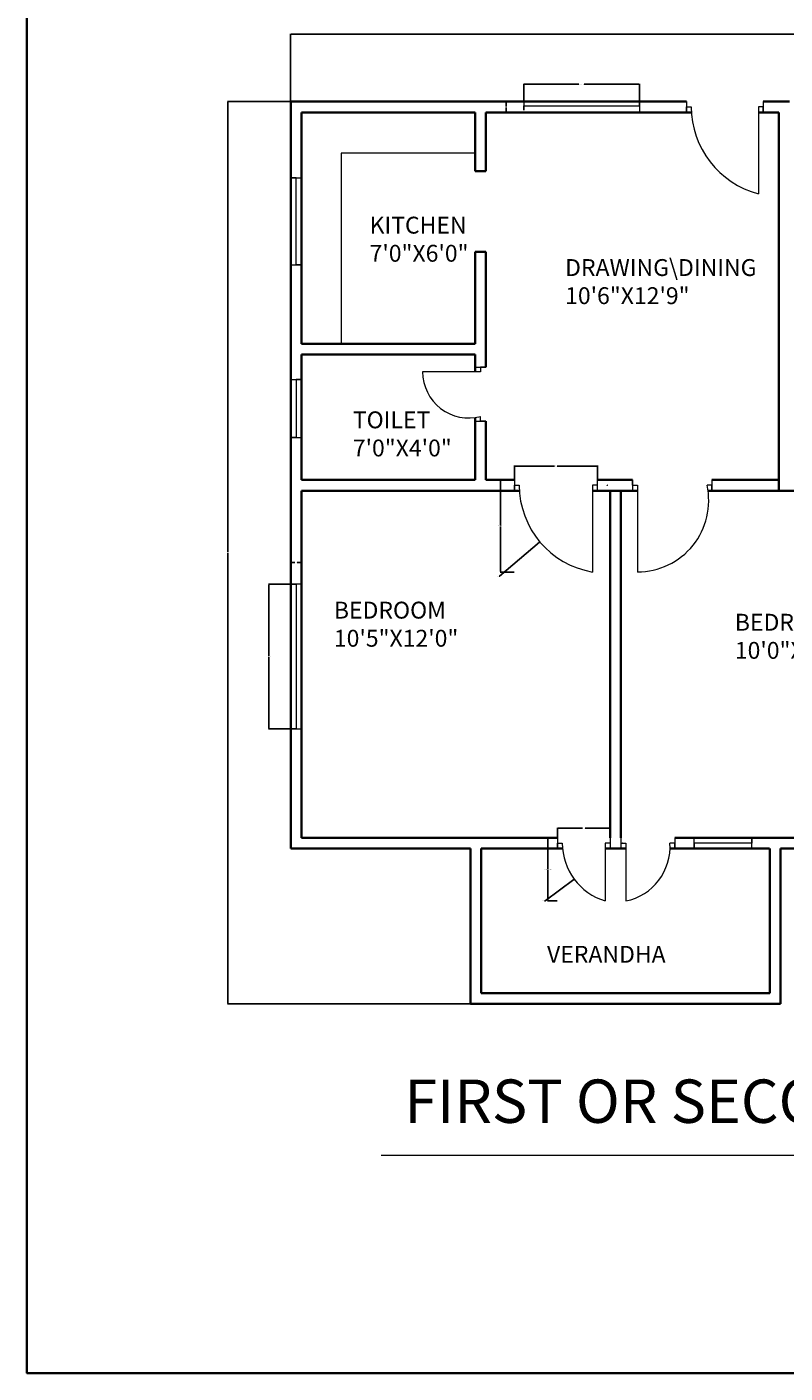
# Model space of a CAD drawing. Units: inches. Extents: x 2055 to 3558, y 1520 to 2888.
# Tile 1 of 8: x 2055 to 2369, y 1520 to 2079. Entities that reach past the tile are written whole.
import ezdxf

# ---------------------------------------------------------------- set-up
doc = ezdxf.new("R2010")
doc.units = ezdxf.units.IN
for name, color, linetype, lineweight in [('A-ANNO-DIMS', 2, 'Continuous', 18), ('A-ANNO-TEXT', 7, 'Continuous', 18), ('A-ANNO-TTLB', 7, 'Continuous', 35), ('A-AREA-IDEN', 7, 'Continuous', 18), ('A-DOOR', 3, 'Continuous', 18), ('A-FLOR-FIXT', 8, 'Continuous', 18), ('A-GLAZ', 4, 'Continuous', 18), ('A-WALL', 7, 'Continuous', 35)]:
    doc.layers.add(name, color=color, linetype=linetype, lineweight=lineweight)
doc.styles.get("Standard").update_dxf_attribs({"font": 'arial.ttf'})
doc.dimstyles.get("Standard").update_dxf_attribs({"dimtxt": 0.18, "dimasz": 0.18, "dimexe": 0.18, "dimexo": 0.0625, "dimgap": 0.09, "dimtad": 0, "dimtih": 1, "dimtoh": 1, "dimdec": 4, "dimzin": 0, "dimdsep": 46, "dimtxsty": 'Standard', "dimcen": 0.09, "dimadec": 0, "dimazin": 0, "dimtfac": 1, "dimtdec": 4, "dimtofl": 0, "dimtmove": 0, "dimatfit": 3, "dimfxl": 1, "dimtolj": 1, "dimtzin": 0, "dimarcsym": 0})

# ---------------------------------------------------------------- blocks, each defined once
blk = doc.blocks.new('DOOR-ENTRY-36-C')
for p, q in [((0, 38.25), (0, 33.75)), ((0, 33.75), (0, 36)), ((0, 36), (2, 36)), ((31.88, 36), (29.88, 36)), ((29.88, 36), (29.88, 0)), ((31.88, 38.25), (31.88, 33.75)), ((31.88, 33.75), (31.88, 36))]:
    blk.add_line(p, q)
blk.add_arc((39.18, 36), 37.18, 180, 255.5126)
blk = doc.blocks.new('DOOR-BATH-24-C')
for p, q in [((21.75, 22.46), (26.25, 22.46)), ((26.25, 22.46), (24, 22.46)), ((24, 22.46), (24, 20.46)), ((24, 20.46), (0, 20.46)), ((24, 0), (24, 2)), ((21.75, 0), (26.25, 0)), ((26.25, 0), (24, 0))]:
    blk.add_line(p, q)
blk.add_arc((19.1, 20.46), 19.1, 180, 284.8648)
blk = doc.blocks.new('DOOR-BED-36-D')
for p, q in [((0.16, 33.75), (0, 38.25)), ((0, 38.25), (0.08, 36)), ((0.08, 36), (2.08, 36)), ((2.08, 36), (2.08, 0)), ((33, 36), (31, 36)), ((33, 38.25), (33, 33.75)), ((33, 33.75), (33, 36))]:
    blk.add_line(p, q)
blk.add_arc((2.08, 29.62), 29.61, 270, 12.4519)
blk = doc.blocks.new('DOOR-BED-36-E')
for p, q in [((0, 38.25), (0, 33.75)), ((0, 33.75), (0, 36)), ((0, 36), (2, 36)), ((34.42, 36), (32.42, 36)), ((32.42, 36), (32.42, 0)), ((34.42, 33.75), (34.42, 38.25))]:
    blk.add_line(p, q)
blk.add_arc((38.51, 36), 36.51, 180, 260.3872)
blk = doc.blocks.new('DOOR-VERANDA-24-C')
for p, q in [((0, 26.25), (0, 21.75)), ((0, 21.75), (0, 24)), ((0, 24), (2, 24)), ((21.82, 24), (19.82, 24)), ((19.82, 24), (19.82, 0)), ((21.82, 26.25), (21.82, 21.75))]:
    blk.add_line(p, q)
blk.add_arc((27.07, 24), 25.07, 180, 253.1988)
blk = doc.blocks.new('DOOR-VERANDA-24-D')
for p, q in [((0, 26.25), (0, 21.75)), ((0, 24), (2, 24)), ((2, 24), (2, 0)), ((22.33, 24), (20.33, 24)), ((22.33, 26.25), (22.33, 21.75)), ((22.33, 21.75), (22.33, 24))]:
    blk.add_line(p, q)
blk.add_arc((-2.55, 22.48), 22.94, 281.4505, 3.8037)
blk = doc.blocks.new('WIN-36')
for p, q in [((2.25, 36), (0, 36)), ((0, 36), (4.5, 36)), ((2.25, 0), (2.25, 36)), ((0, 0), (4.5, 0)), ((4.5, 0), (2.25, 0))]:
    blk.add_line(p, q)
blk = doc.blocks.new('WIN-24')
for p, q in [((0, 24), (4.5, 24)), ((4.5, 24), (2.25, 24)), ((2.25, 24), (2.25, 0)), ((2.25, 0), (0, 0)), ((0, 0), (4.5, 0))]:
    blk.add_line(p, q)
blk = doc.blocks.new('WIN-60-2')
for p, q in [((4.5, 60), (0, 60)), ((0, 60), (2.25, 60)), ((2.25, 60), (2.25, 0)), ((2.25, 0), (0, 0)), ((0, 0), (4.5, 0))]:
    blk.add_line(p, q)
blk = doc.blocks.new('WIN-48-2')
for p, q in [((0, 4.5), (0, 0.97)), ((0, 0.97), (0, 2.74)), ((0, 2.74), (48, 2.74)), ((48, 2.74), (48, 4.5)), ((48, 4.5), (48, 0))]:
    blk.add_line(p, q)
blk = doc.blocks.new('COUNTER-3')
for p, q in [((55.49, 79.01), (0, 79.01)), ((0, 79.01), (0, 0))]:
    blk.add_line(p, q)
blk = doc.blocks.new('VERANDA-PERIMETER')
for p, q in [((0, 0), (0, 64.5)), ((4.5, 64.5), (4.5, 4.5)), ((124.15, 4.5), (124.15, 64.5)), ((128.65, 64.5), (128.65, 4.5)), ((4.5, 0), (0, 0)), ((4.5, 4.5), (124.15, 4.5)), ((128.65, 0), (4.5, 0)), ((128.65, 4.5), (128.65, 0))]:
    blk.add_line(p, q)
blk = doc.blocks.new('*D48')
at = {"layer": 'A-ANNO-DIMS', "color": 0, "lineweight": -2, "transparency": 16777216}
for p, q in [((2164.11, 1847.67), (2154.99, 1847.67)), ((2155.17, 1847.49), (2155.17, 1817.85)), ((2155.17, 1787.85), (2155.17, 1817.48)), ((2164.11, 1787.67), (2154.99, 1787.67))]:
    blk.add_line(p, q, dxfattribs=at)
at = {"layer": 'A-ANNO-DIMS', "color": 0, "transparency": 16777216}
for points in [[(2155.14, 1847.49), (2155.2, 1847.49), (2155.17, 1847.67)], [(2155.14, 1787.85), (2155.2, 1787.85), (2155.17, 1787.67)]]:
    blk.add_solid(points, dxfattribs=at)
at = {"layer": 'Defpoints', "color": 0, "transparency": 16777216}
for p in [(2155.17, 1847.67), (2164.17, 1847.67), (2164.17, 1787.67)]:
    blk.add_point(p, dxfattribs=at)
at = {"layer": 'A-ANNO-DIMS', "color": 0, "transparency": 16777216, "insert": (2155.17, 1817.67), "char_height": 0.18, "attachment_point": 5}
blk.add_mtext('\\A1;WINDOW 60 TYP.', dxfattribs=at)
blk = doc.blocks.new('*D49')
at = {"layer": 'A-ANNO-DIMS', "color": 0, "lineweight": -2, "transparency": 16777216}
for p, q in [((2164.17, 1847.73), (2164.17, 1856.85)), ((2164.35, 1856.67), (2165.97, 1856.67)), ((2168.49, 1856.67), (2166.88, 1856.67)), ((2168.67, 1847.73), (2168.67, 1856.85))]:
    blk.add_line(p, q, dxfattribs=at)
at = {"layer": 'A-ANNO-DIMS', "color": 0, "transparency": 16777216}
for points in [[(2164.35, 1856.7), (2164.35, 1856.64), (2164.17, 1856.67)], [(2168.49, 1856.7), (2168.49, 1856.64), (2168.67, 1856.67)]]:
    blk.add_solid(points, dxfattribs=at)
at = {"layer": 'Defpoints', "color": 0, "transparency": 16777216}
for p in [(2168.67, 1856.67), (2164.17, 1847.67), (2168.67, 1847.67)]:
    blk.add_point(p, dxfattribs=at)
at = {"layer": 'A-ANNO-DIMS', "color": 0, "transparency": 16777216, "insert": (2166.42, 1856.67), "char_height": 0.18, "attachment_point": 5}
blk.add_mtext('\\A1;5 TYP.', dxfattribs=at)
blk = doc.blocks.new('*D76')
at = {"layer": 'A-ANNO-DIMS', "color": 0, "lineweight": -2, "transparency": 16777216}
for p, q in [((2256.93, 1891), (2251.07, 1891)), ((2251.25, 1890.82), (2251.25, 1872.06)), ((2251.25, 1852.93), (2251.25, 1871.69)), ((2256.93, 1852.75), (2251.07, 1852.75))]:
    blk.add_line(p, q, dxfattribs=at)
at = {"layer": 'A-ANNO-DIMS', "color": 0, "transparency": 16777216}
for points in [[(2251.22, 1890.82), (2251.28, 1890.82), (2251.25, 1891)], [(2251.22, 1852.93), (2251.28, 1852.93), (2251.25, 1852.75)]]:
    blk.add_solid(points, dxfattribs=at)
at = {"layer": 'Defpoints', "color": 0, "transparency": 16777216}
for p in [(2251.25, 1891), (2256.99, 1891), (2256.99, 1852.75)]:
    blk.add_point(p, dxfattribs=at)
at = {"layer": 'A-ANNO-DIMS', "color": 0, "transparency": 16777216, "insert": (2251.25, 1871.87), "char_height": 0.18, "attachment_point": 5}
blk.add_mtext('\\A1;BED DOOR 38 TYP.', dxfattribs=at)
blk = doc.blocks.new('*D77')
at = {"layer": 'A-ANNO-DIMS', "color": 0, "lineweight": -2, "transparency": 16777216}
for p, q in [((2256.99, 1891.06), (2256.99, 1896.92)), ((2257.17, 1896.74), (2273.67, 1896.74)), ((2291.23, 1896.74), (2274.73, 1896.74)), ((2291.41, 1891.06), (2291.41, 1896.92))]:
    blk.add_line(p, q, dxfattribs=at)
at = {"layer": 'A-ANNO-DIMS', "color": 0, "transparency": 16777216}
for points in [[(2257.17, 1896.77), (2257.17, 1896.71), (2256.99, 1896.74)], [(2291.23, 1896.77), (2291.23, 1896.71), (2291.41, 1896.74)]]:
    blk.add_solid(points, dxfattribs=at)
at = {"layer": 'Defpoints', "color": 0, "transparency": 16777216}
for p in [(2291.41, 1896.74), (2256.99, 1891), (2291.41, 1891)]:
    blk.add_point(p, dxfattribs=at)
at = {"layer": 'A-ANNO-DIMS', "color": 0, "transparency": 16777216, "insert": (2274.2, 1896.74), "char_height": 0.18, "attachment_point": 5}
blk.add_mtext('\\A1;34 TYP.', dxfattribs=at)
blk = doc.blocks.new('*D86')
at = {"layer": 'A-ANNO-DIMS', "color": 0, "lineweight": -2, "transparency": 16777216}
for p, q in [((2274.79, 1742.5), (2270.73, 1742.5)), ((2270.91, 1742.32), (2270.91, 1729.56)), ((2270.91, 1716.43), (2270.91, 1729.19)), ((2274.79, 1716.25), (2270.73, 1716.25))]:
    blk.add_line(p, q, dxfattribs=at)
at = {"layer": 'A-ANNO-DIMS', "color": 0, "transparency": 16777216}
for points in [[(2270.88, 1742.32), (2270.94, 1742.32), (2270.91, 1742.5)], [(2270.88, 1716.43), (2270.94, 1716.43), (2270.91, 1716.25)]]:
    blk.add_solid(points, dxfattribs=at)
at = {"layer": 'Defpoints', "color": 0, "transparency": 16777216}
for p in [(2270.91, 1742.5), (2274.85, 1742.5), (2274.85, 1716.25)]:
    blk.add_point(p, dxfattribs=at)
at = {"layer": 'A-ANNO-DIMS', "color": 0, "transparency": 16777216, "insert": (2270.91, 1729.37), "char_height": 0.18, "attachment_point": 5}
blk.add_mtext('\\A1;VERANDA DOOR 26 TYP.', dxfattribs=at)
blk = doc.blocks.new('*D87')
at = {"layer": 'A-ANNO-DIMS', "color": 0, "lineweight": -2, "transparency": 16777216}
for p, q in [((2274.85, 1742.56), (2274.85, 1746.62)), ((2275.03, 1746.44), (2285.23, 1746.44)), ((2296.49, 1746.44), (2286.29, 1746.44)), ((2296.67, 1742.56), (2296.67, 1746.62))]:
    blk.add_line(p, q, dxfattribs=at)
at = {"layer": 'A-ANNO-DIMS', "color": 0, "transparency": 16777216}
for points in [[(2275.03, 1746.47), (2275.03, 1746.41), (2274.85, 1746.44)], [(2296.49, 1746.47), (2296.49, 1746.41), (2296.67, 1746.44)]]:
    blk.add_solid(points, dxfattribs=at)
at = {"layer": 'Defpoints', "color": 0, "transparency": 16777216}
for p in [(2296.67, 1746.44), (2274.85, 1742.5), (2296.67, 1742.5)]:
    blk.add_point(p, dxfattribs=at)
at = {"layer": 'A-ANNO-DIMS', "color": 0, "transparency": 16777216, "insert": (2285.76, 1746.44), "char_height": 0.18, "attachment_point": 5}
blk.add_mtext('\\A1;22 TYP.', dxfattribs=at)
blk = doc.blocks.new('*D104')
at = {"layer": 'A-ANNO-DIMS', "color": 0, "lineweight": -2, "transparency": 16777216}
for p, q in [((2260.84, 2048.06), (2260.84, 2055.38)), ((2261.02, 2055.2), (2283.72, 2055.2)), ((2308.66, 2055.2), (2285.96, 2055.2)), ((2308.84, 2048.06), (2308.84, 2055.38))]:
    blk.add_line(p, q, dxfattribs=at)
at = {"layer": 'A-ANNO-DIMS', "color": 0, "transparency": 16777216}
for points in [[(2261.02, 2055.23), (2261.02, 2055.17), (2260.84, 2055.2)], [(2308.66, 2055.23), (2308.66, 2055.17), (2308.84, 2055.2)]]:
    blk.add_solid(points, dxfattribs=at)
at = {"layer": 'Defpoints', "color": 0, "transparency": 16777216}
for p in [(2308.84, 2055.2), (2260.84, 2048), (2308.84, 2048)]:
    blk.add_point(p, dxfattribs=at)
at = {"layer": 'A-ANNO-DIMS', "color": 0, "transparency": 16777216, "insert": (2284.84, 2055.2), "char_height": 0.18, "attachment_point": 5}
blk.add_mtext('\\A1;WINDOW 48 TYP.', dxfattribs=at)
blk = doc.blocks.new('*D105')
at = {"layer": 'A-ANNO-DIMS', "color": 0, "lineweight": -2, "transparency": 16777216}
for p, q in [((2260.77, 2048), (2253.46, 2048)), ((2253.64, 2047.82), (2253.64, 2045.93)), ((2253.64, 2043.68), (2253.64, 2045.57)), ((2260.77, 2043.5), (2253.46, 2043.5))]:
    blk.add_line(p, q, dxfattribs=at)
at = {"layer": 'A-ANNO-DIMS', "color": 0, "transparency": 16777216}
for points in [[(2253.61, 2047.82), (2253.67, 2047.82), (2253.64, 2048)], [(2253.61, 2043.68), (2253.67, 2043.68), (2253.64, 2043.5)]]:
    blk.add_solid(points, dxfattribs=at)
at = {"layer": 'Defpoints', "color": 0, "transparency": 16777216}
for p in [(2253.64, 2048), (2260.84, 2048), (2260.84, 2043.5)]:
    blk.add_point(p, dxfattribs=at)
at = {"layer": 'A-ANNO-DIMS', "color": 0, "transparency": 16777216, "insert": (2253.64, 2045.75), "char_height": 0.18, "attachment_point": 5}
blk.add_mtext('\\A1;5 TYP.', dxfattribs=at)
blk = doc.blocks.new('*D121')
at = {"layer": 'A-ANNO-DIMS', "color": 0, "lineweight": -2, "transparency": 16777216}
for p, q in [((2164.17, 2048.06), (2164.17, 2076.13)), ((2164.35, 2075.95), (2420.03, 2075.95)), ((2676.49, 2075.95), (2420.82, 2075.95)), ((2676.67, 2048.06), (2676.67, 2076.13))]:
    blk.add_line(p, q, dxfattribs=at)
at = {"layer": 'A-ANNO-DIMS', "color": 0, "transparency": 16777216}
for points in [[(2164.35, 2075.98), (2164.35, 2075.92), (2164.17, 2075.95)], [(2676.49, 2075.98), (2676.49, 2075.92), (2676.67, 2075.95)]]:
    blk.add_solid(points, dxfattribs=at)
at = {"layer": 'Defpoints', "color": 0, "transparency": 16777216}
for p in [(2676.67, 2075.95), (2164.17, 2048), (2676.67, 2048)]:
    blk.add_point(p, dxfattribs=at)
at = {"layer": 'A-ANNO-DIMS', "color": 0, "transparency": 16777216, "insert": (2420.42, 2075.95), "char_height": 0.18, "attachment_point": 5}
blk.add_mtext('\\A1;512.5', dxfattribs=at)
blk = doc.blocks.new('*D122')
at = {"layer": 'A-ANNO-DIMS', "color": 0, "lineweight": -2, "transparency": 16777216}
for p, q in [((2164.11, 2048), (2137.94, 2048)), ((2138.12, 2047.82), (2138.12, 1860.93)), ((2138.12, 1673.68), (2138.12, 1860.57)), ((2238.68, 1673.5), (2137.94, 1673.5))]:
    blk.add_line(p, q, dxfattribs=at)
at = {"layer": 'A-ANNO-DIMS', "color": 0, "transparency": 16777216}
for points in [[(2138.09, 2047.82), (2138.15, 2047.82), (2138.12, 2048)], [(2138.09, 1673.68), (2138.15, 1673.68), (2138.12, 1673.5)]]:
    blk.add_solid(points, dxfattribs=at)
at = {"layer": 'Defpoints', "color": 0, "transparency": 16777216}
for p in [(2164.17, 2048), (2138.12, 1673.5), (2238.74, 1673.5)]:
    blk.add_point(p, dxfattribs=at)
at = {"layer": 'A-ANNO-DIMS', "color": 0, "transparency": 16777216, "insert": (2138.12, 1860.75), "char_height": 0.18, "attachment_point": 5}
blk.add_mtext('\\A1;374.5', dxfattribs=at)
blk = doc.blocks.new('*D174')
at = {"layer": 'A-ANNO-DIMS', "color": 0, "lineweight": -2, "transparency": 16777216}
for p, q in [((2295.41, 1888.75), (2295.59, 1888.75)), ((2295.5, 1888.66), (2295.5, 1888.84)), ((2250.88, 1851.05), (2267.47, 1865.07)), ((2250.7, 1851.05), (2250.88, 1851.05))]:
    blk.add_line(p, q, dxfattribs=at)
at = {"layer": 'A-ANNO-DIMS', "color": 0, "transparency": 16777216}
blk.add_solid([(2267.46, 1865.09), (2267.49, 1865.05), (2267.61, 1865.18)], dxfattribs=at)
at = {"layer": 'Defpoints', "color": 0, "transparency": 16777216}
for p in [(2295.5, 1888.75), (2267.61, 1865.18)]:
    blk.add_point(p, dxfattribs=at)
at = {"layer": 'A-ANNO-DIMS', "color": 0, "transparency": 16777216, "insert": (2250.24, 1851.05), "char_height": 0.18, "attachment_point": 5}
blk.add_mtext('\\A1;R36.51', dxfattribs=at)
blk = doc.blocks.new('*D180')
at = {"layer": 'A-ANNO-DIMS', "color": 0, "lineweight": -2, "transparency": 16777216}
for p, q in [((2301.83, 1740.25), (2302.01, 1740.25)), ((2301.92, 1740.16), (2301.92, 1740.34)), ((2269.72, 1716.33), (2281.65, 1725.19)), ((2269.54, 1716.33), (2269.72, 1716.33))]:
    blk.add_line(p, q, dxfattribs=at)
at = {"layer": 'A-ANNO-DIMS', "color": 0, "transparency": 16777216}
blk.add_solid([(2281.63, 1725.22), (2281.67, 1725.17), (2281.79, 1725.3)], dxfattribs=at)
at = {"layer": 'Defpoints', "color": 0, "transparency": 16777216}
for p in [(2301.92, 1740.25), (2281.79, 1725.3)]:
    blk.add_point(p, dxfattribs=at)
at = {"layer": 'A-ANNO-DIMS', "color": 0, "transparency": 16777216, "insert": (2269.06, 1716.33), "char_height": 0.18, "attachment_point": 5}
blk.add_mtext('\\A1;R25.07', dxfattribs=at)

msp = doc.modelspace()

# ---------------------------------------------------------------- linework, layer by layer
at = {"layer": 'A-ANNO-TEXT'}
msp.add_line((2201.7713, 1610.7234), (2548.8845, 1610.7234), dxfattribs=at)
at = {"layer": 'A-ANNO-TTLB'}
msp.add_lwpolyline([(2054.7598, 2888.2545), (3557.8479, 2888.2545), (3557.8479, 1520.3256), (2054.7598, 1520.3256)], close=True, dxfattribs=at)
at = {"layer": 'A-WALL'}
for p, q in [((2164.1747, 2047.9995), (2328.3753, 2047.9995)), ((2164.1747, 2047.9995), (2164.1747, 1737.9995)), ((2360.2558, 2047.9995), (2371.1747, 2047.9995)), ((2168.6747, 2043.4995), (2168.6747, 1947.4995)), ((2168.6747, 2043.4995), (2240.6747, 2043.4995)), ((2240.6747, 2043.4995), (2240.6747, 2019.1081)), ((2245.1747, 2043.4995), (2245.1747, 2019.1081)), ((2245.1747, 2043.4995), (2330.4434, 2043.4995)), ((2358.2558, 2043.4995), (2366.6747, 2043.4995)), ((2366.6747, 2043.4995), (2366.6747, 1947.4995)), ((2366.6747, 2043.4995), (2366.6747, 1886.4995)), ((2240.6747, 2019.1081), (2245.1747, 2019.1081)), ((2245.1747, 1985.6374), (2240.6747, 1985.6374)), ((2240.6747, 1985.6374), (2240.6747, 1947.4995)), ((2245.1747, 1985.6374), (2245.1747, 1937.7895)), ((2168.6747, 1947.4995), (2240.6747, 1947.4995)), ((2168.6747, 1942.9995), (2240.6747, 1942.9995)), ((2168.6747, 1942.9995), (2168.6747, 1890.9995)), ((2240.6747, 1942.9995), (2240.6747, 1935.7895)), ((2240.6747, 1916.8741), (2240.6747, 1890.9995)), ((2245.1747, 1915.3286), (2245.1747, 1890.9995)), ((2168.6747, 1890.9995), (2240.6747, 1890.9995)), ((2245.1747, 1890.9995), (2256.9898, 1890.9995)), ((2291.4053, 1890.9995), (2305.9247, 1890.9995)), ((2338.9237, 1890.9995), (2366.6747, 1890.9995)), ((2168.6747, 1886.4995), (2259.0592, 1886.4995)), ((2168.6747, 1886.4995), (2168.6747, 1742.4995)), ((2245.1747, 1886.4995), (2259.0592, 1886.4995)), ((2289.4053, 1886.4995), (2308.0058, 1886.4995)), ((2289.4053, 1886.4995), (2308.0058, 1886.4995)), ((2296.6747, 1886.4995), (2296.6747, 1742.4995)), ((2301.1747, 1886.4995), (2301.1747, 1742.4995)), ((2337.3301, 1886.4995), (2366.6747, 1886.4995)), ((2337.3301, 1886.4995), (2422.6747, 1886.4995)), ((2164.1747, 1737.9995), (2238.745, 1737.9995)), ((2168.6747, 1742.4995), (2274.8511, 1742.4995)), ((2243.245, 1737.9995), (2276.9523, 1737.9995)), ((2245.1747, 1742.4995), (2274.8511, 1742.4995)), ((2294.6747, 1737.9995), (2303.1747, 1737.9995)), ((2321.545, 1737.9995), (2362.8911, 1737.9995)), ((2323.5061, 1742.4995), (2508.8547, 1742.4995)), ((2323.5061, 1742.4995), (2366.6747, 1742.4995)), ((2367.3911, 1737.9995), (2422.6747, 1737.9995))]:
    msp.add_line(p, q, dxfattribs=at)

# ---------------------------------------------------------------- block references
at = {"layer": 'A-DOOR'}
for name, p in [('DOOR-ENTRY-36-C', (2328.375, 2009.749)), ('DOOR-BATH-24-C', (2218.925, 1915.329)), ('DOOR-BED-36-E', (2256.99, 1852.749)), ('DOOR-BED-36-D', (2305.925, 1852.749)), ('DOOR-VERANDA-24-C', (2274.851, 1716.249)), ('DOOR-VERANDA-24-D', (2301.175, 1716.249))]:
    msp.add_blockref(name, p, dxfattribs=at)
at = {"layer": 'A-FLOR-FIXT'}
msp.add_blockref('COUNTER-3', (2185.186, 1947.499), dxfattribs=at)
at = {"layer": 'A-GLAZ'}
for name, p in [('WIN-48-2', (2260.837, 2043.499)), ('WIN-36', (2164.175, 1980.291)), ('WIN-24', (2164.175, 1908.63)), ('WIN-60-2', (2164.175, 1787.665))]:
    msp.add_blockref(name, p, dxfattribs=at)
at = {"layer": 'A-GLAZ', "extrusion": (0, 0, -1), "zscale": -1, "rotation": 90}
msp.add_blockref('WIN-24', (-2331.5394, 1737.9998), dxfattribs=at)
at = {"layer": 'A-WALL'}
msp.add_blockref('VERANDA-PERIMETER', (2238.745, 1673.499), dxfattribs=at)

# ---------------------------------------------------------------- texts
at = {"layer": 'A-ANNO-TEXT', "insert": (2211.3331, 1642.1482), "char_height": 18, "attachment_point": 1}
msp.add_mtext_dynamic_manual_height_columns('FIRST OR SECOND FLOOR ', width=532.043788, gutter_width=12.5, heights=[0], dxfattribs=at)
at = {"layer": 'A-AREA-IDEN', "char_height": 7, "attachment_point": 1}
for s, width, insert in [('KITCHEN\\P7\'0"X6\'0"', 92.673757, (2196.9206, 2000.1878)), ('DRAWING\\\\DINING\\P10\'6"X12\'9"', 76.318653, (2278.0286, 1982.594)), ('TOILET\\P7\'0"X4\'0"', 58.820839, (2189.9617, 1919.3885)), ('BEDROOM\\P10\'5"X12\'0"', 285.522885, (2182.0987, 1840.4245)), ('BEDROOM\\P10\'0"X12\'0"', 113.389445, (2348.4409, 1835.3994)), ('VERANDHA', 73.975505, (2270.5238, 1697.6201))]:
    msp.add_mtext_dynamic_manual_height_columns(s, width=width, gutter_width=12.5, heights=[0], dxfattribs=dict(at, insert=insert))

# ---------------------------------------------------------------- dimensions: what is measured, and where the dimension line sits
at = {"layer": 'A-ANNO-DIMS'}
dim = msp.add_linear_dim(base=(2676.6747, 2075.9495), p1=(2164.1747, 2047.9995), p2=(2676.6747, 2047.9995), dimstyle='Standard', override={"dimdec": 1, "dimlfac": 1, "dimrnd": 0, "dimzin": 0, "dimdsep": 46, "dimlunit": 2}, dxfattribs=at)
dim.commit()
dim.dimension.update_dxf_attribs({"geometry": '*D121', "text_midpoint": (2420.4247, 2075.9495)})
for base, p1, p2, text, picture, middle in [((2308.8371, 2055.1995), (2260.8371, 2047.9995), (2308.8371, 2047.9995), 'WINDOW <> TYP.', '*D104', (2284.8371, 2055.1995)), ((2291.4053, 1896.737), (2256.9898, 1890.9995), (2291.4053, 1890.9995), '<> TYP.', '*D77', (2274.1976, 1896.737)), ((2168.6746671216, 1856.6650679317), (2164.1746671216, 1847.6650679317), (2168.6746671216, 1847.6650679317), '<> TYP.', '*D49', (2166.4246671216, 1856.6650679317)), ((2296.6747, 1746.437), (2274.8511, 1742.4995), (2296.6747, 1742.4995), '<> TYP.', '*D87', (2285.7629, 1746.437))]:
    dim = msp.add_linear_dim(base=base, p1=p1, p2=p2, text=text, dimstyle='Standard', override={"dimdec": 0, "dimlfac": 1, "dimrnd": 0, "dimzin": 0, "dimdsep": 46, "dimlunit": 2}, dxfattribs=at)
    dim.commit()
    dim.dimension.update_dxf_attribs({"geometry": picture, "text_midpoint": middle})
dim = msp.add_linear_dim(base=(2138.1247, 1673.4995), p1=(2164.1747, 2047.9995), p2=(2238.745, 1673.4995), angle=90, dimstyle='Standard', override={"dimdec": 1, "dimlfac": 1, "dimrnd": 0, "dimzin": 0, "dimdsep": 46, "dimlunit": 2}, dxfattribs=at)
dim.commit()
dim.dimension.update_dxf_attribs({"geometry": '*D122', "text_midpoint": (2138.1247, 1860.7495)})
for base, p1, p2, text, picture, middle in [((2253.6370693542, 2047.9994988353), (2260.8370693542, 2043.4994988353), (2260.8370693542, 2047.9994988353), '<> TYP.', '*D105', (2253.6370693542, 2045.7494988353)), ((2251.2523, 1890.9995), (2256.9898, 1852.7495), (2256.9898, 1890.9995), 'BED DOOR <> TYP.', '*D76', (2251.2523, 1871.8745)), ((2155.1747, 1847.6651), (2164.1747, 1787.6651), (2164.1747, 1847.6651), 'WINDOW <> TYP.', '*D48', (2155.1747, 1817.6651)), ((2270.9136, 1742.4995), (2274.8511, 1716.2495), (2274.8511, 1742.4995), 'VERANDA DOOR <> TYP.', '*D86', (2270.9136, 1729.3745))]:
    dim = msp.add_linear_dim(base=base, p1=p1, p2=p2, angle=90, text=text, dimstyle='Standard', override={"dimdec": 0, "dimlfac": 1, "dimrnd": 0, "dimzin": 0, "dimdsep": 46, "dimlunit": 2}, dxfattribs=at)
    dim.commit()
    dim.dimension.update_dxf_attribs({"geometry": picture, "text_midpoint": middle})
for center, mpoint, picture, middle in [((2295.5025, 1888.7495), (2267.6119, 1865.1849), '*D174', (2250.2351, 1851.0462)), ((2301.9213, 1740.2495), (2281.7943, 1725.3022), '*D180', (2269.0584, 1716.3339))]:
    dim = msp.add_radius_dim(center=center, mpoint=mpoint, dimstyle='Standard', override={"dimdec": 2, "dimlfac": 1, "dimrnd": 0, "dimzin": 0, "dimdsep": 46, "dimlunit": 2}, dxfattribs=at)
    dim.commit()
    dim.dimension.update_dxf_attribs({"geometry": picture, "text_midpoint": middle, "dimtype": 164})

doc.saveas('drawing.dxf')
